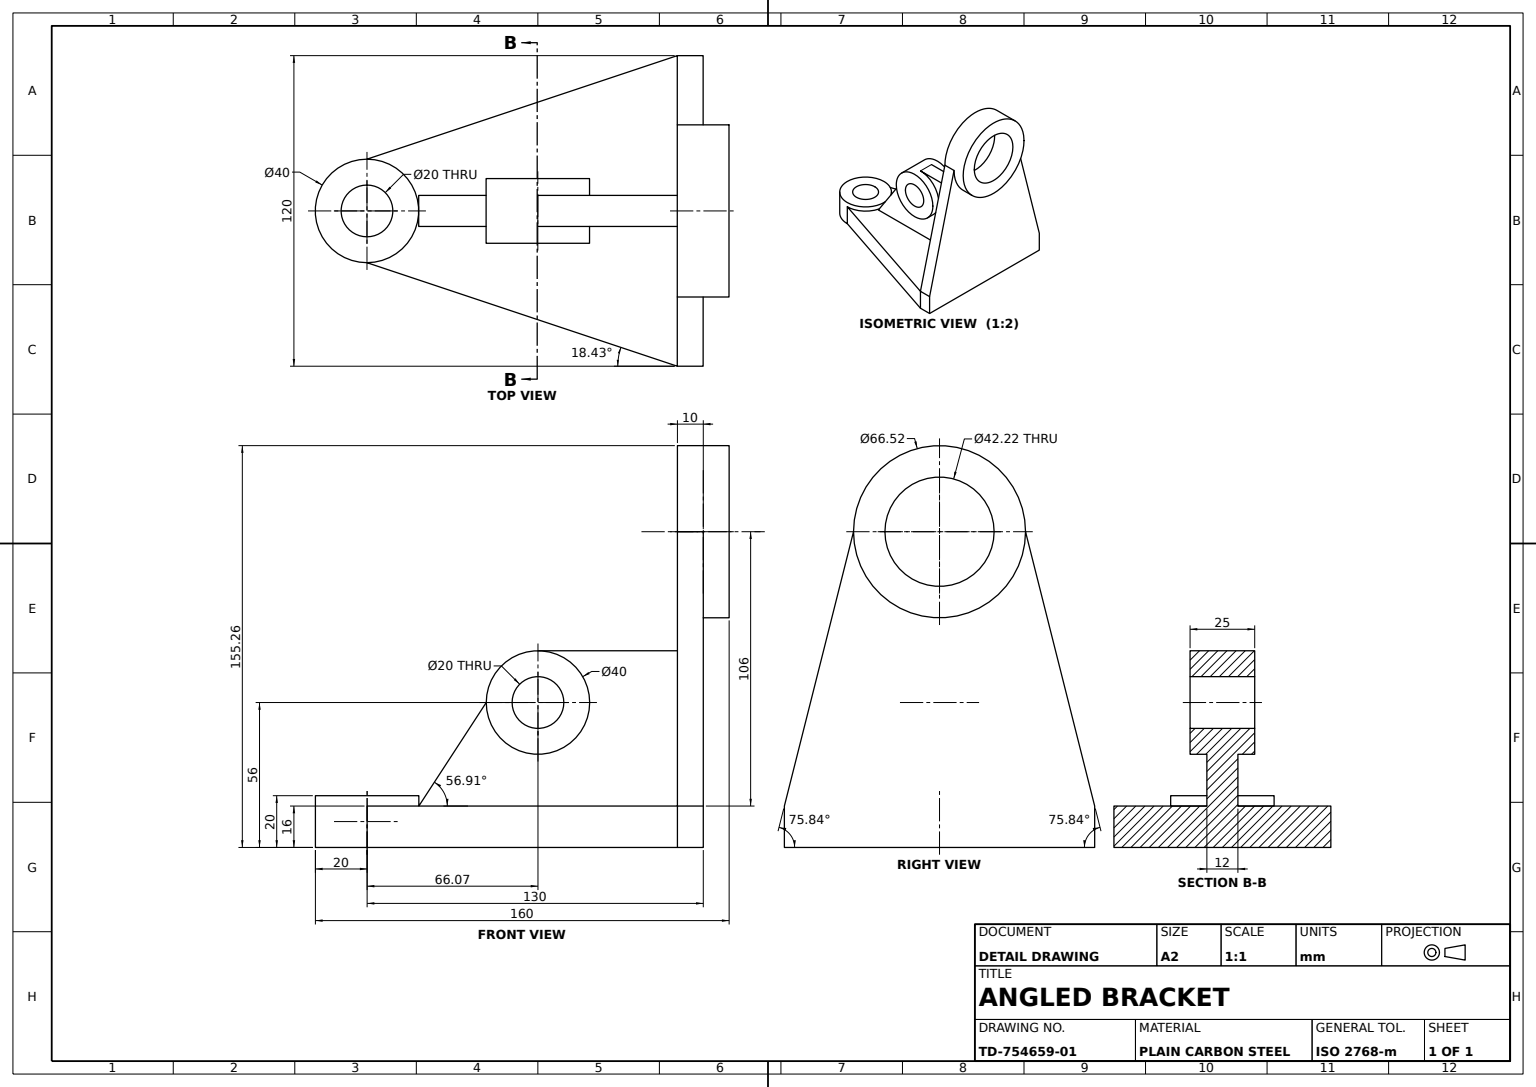
from build123d import *

# Parameters (mm, degrees)
BASE_BOSS_RING_SKETCH_R    = 20
BASE_BOSS_RING_SKETCH_R_2  = 10
BASE_BOSS_RING_40_DEPTH    = 20
BASE_PLATE_DEPTH           = 16
UPPER_BOSS_RING_SKETCH_R   = 33.258405
UPPER_BOSS_RING_SKETCH_R_2 = 21.112311
UPPER_BOSS_RING_DEPTH      = 10
UPRIGHT_WEB_DEPTH          = 10
MIDDLE_BOSS_SKETCH_R       = 20
MIDDLE_BOSS_SKETCH_R_2     = 10
MIDDLE_BOSS_DEPTH          = 12.5
GUSSET_RIB_DEPTH           = 6
MIDDLE_BOSS_BORE_SKETCH_R  = 10
MIDDLE_BOSS_BORE_DEPTH     = 220.228585


with BuildPart() as part:
    # Base Boss Ring Sketch → Base Boss Ring Ø40 (new body)
    with BuildSketch(Plane(origin=(0, 0, 0), x_dir=(1, 0, 0), z_dir=(0, 1, 0))):
        with Locations(Location((0, 0, 0), (0, 0, 270))):
            Circle(BASE_BOSS_RING_SKETCH_R)
        with Locations(Location((0, 0, 0), (0, 0, 270))):
            Circle(BASE_BOSS_RING_SKETCH_R_2, mode=Mode.SUBTRACT)
    extrude(amount=BASE_BOSS_RING_40_DEPTH)

    # Base Plate Sketch → Base Plate (add)
    with BuildSketch(Plane(origin=(0, 0, 0), x_dir=(1, 0, 0), z_dir=(0, 1, 0))):
        with BuildLine():
            Line((120, 60), (130, 60))
            Line((130, 60), (130, -60))
            Line((130, -60), (120, -60))
            Line((120, -60), (0, -20))
            ThreePointArc((0, -20), (20, 0), (0, 20))
            Line((0, 20), (120, 60))
        make_face()
    extrude(amount=BASE_PLATE_DEPTH)



with BuildPart() as body_2:
    # Upper Boss Ring Sketch → Upper Boss Ring (new, symmetric)
    with BuildSketch(Plane(origin=(130, 0, 0), x_dir=(0, 0, -1), z_dir=(1, 0, 0))):
        with Locations((0, 122)):
            Circle(UPPER_BOSS_RING_SKETCH_R)
        with Locations((0, 122)):
            Circle(UPPER_BOSS_RING_SKETCH_R_2, mode=Mode.SUBTRACT)
    extrude(amount=UPPER_BOSS_RING_DEPTH, both=True)


with BuildPart() as part_1:
    add(part.part)

    add(body_2.part)  # Upright Web merges body 2
    # Upright Web Sketch → Upright Web (add)
    with BuildSketch(Plane(origin=(130, 0, 0), x_dir=(0, 0, -1), z_dir=(1, 0, 0))):
        with BuildLine():
            ThreePointArc((-33.258405, 122), (0, 88.741595), (33.258405, 122))
            Line((33.258405, 122), (60, 16))
            Line((60, 16), (-60, 16))
            Line((-60, 16), (-33.258405, 122))
        make_face()
    extrude(amount=-UPRIGHT_WEB_DEPTH)



with BuildPart() as body_2_2:
    # Middle Boss Sketch → Middle Boss (new, symmetric)
    with BuildSketch(Plane.XY):
        with Locations((66.07, 56)):
            Circle(MIDDLE_BOSS_SKETCH_R)
        with Locations((66.07, 56)):
            Circle(MIDDLE_BOSS_SKETCH_R_2, mode=Mode.SUBTRACT)
    extrude(amount=MIDDLE_BOSS_DEPTH, both=True)


with BuildPart() as part_2:
    add(part_1.part)

    add(body_2_2.part)  # Gusset Rib merges body 2 2
    # Gusset Rib Sketch → Gusset Rib (add, symmetric)
    with BuildSketch(Plane.XY):
        with BuildLine():
            Line((66.07, 76), (120, 76))
            Line((120, 76), (120, 16))
            Line((120, 16), (20, 16))
            Line((20, 16), (46.07, 56))
            ThreePointArc((46.07, 56), (51.927864, 70.142136), (66.07, 76))
        make_face()
    extrude(amount=GUSSET_RIB_DEPTH, both=True)

    # Middle Boss Bore Sketch → Middle Boss Bore (cut, through all)
    with BuildSketch(Plane.XY.offset(6)):
        with Locations((66.07, 56)):
            Circle(MIDDLE_BOSS_BORE_SKETCH_R)
    extrude(amount=-MIDDLE_BOSS_BORE_DEPTH, mode=Mode.SUBTRACT)


solid = part_2.part
